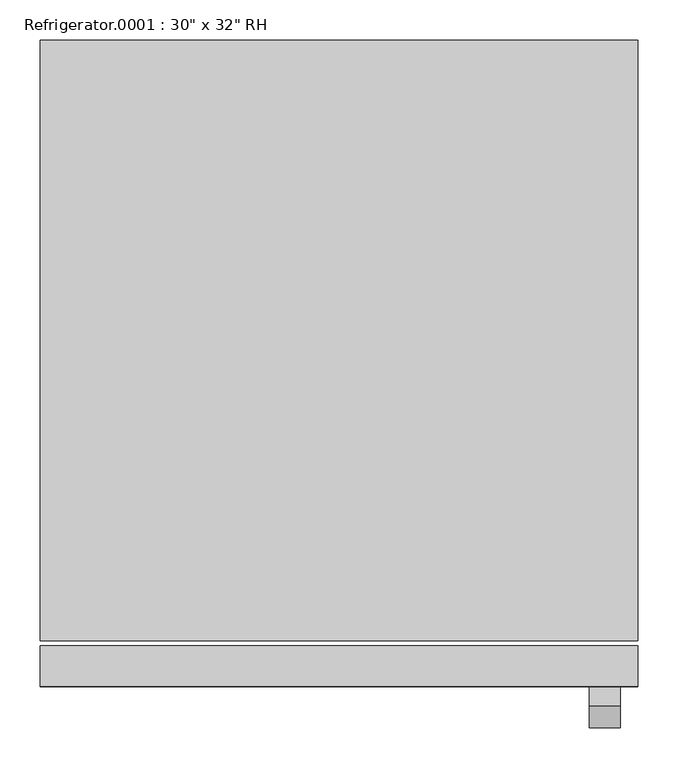
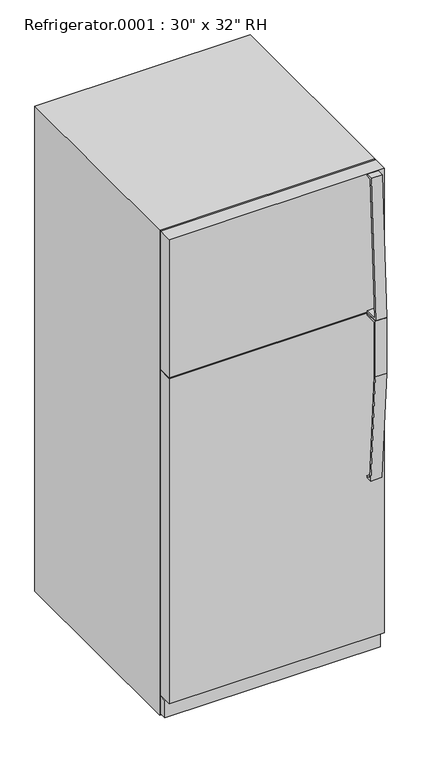
"""IFC4 building model written with IfcOpenShell, lengths in millimetres: proxy geometry."""

from ifc_helpers import new_model, si_unit, frame, origin, origin_with_axes, place, context, project, spatial, polyline, outline, extrude, source, transform, mapped, element, save


def proxy_a13a33b2(model_context):
    return source(origin(), model_context, "Body", "SweptSolid", [
        extrude(outline(polyline([(-417.9010285, 1262.0625), (-462.3510285, 1262.0625), (-462.3510285, 1065.4342469), (-434.8723987, 672.4715334), (-417.9010285, 672.4715334), (-417.9010285, 666.1370017), (-440.7949512, 666.1370017), (-468.7010285, 1065.2125), (-468.7010285, 1268.4125), (-417.9010285, 1268.4125), (-417.9010285, 1262.0625)])), frame((312.7375, 0.0, 0.0), z_axis=(1.0, 0.0, 0.0), x_axis=(0.0, 1.0, 0.0)), (0.0, 0.0, 1.0), 38.4332978),
        extrude(outline(polyline([(-442.739413, 1778.0), (-418.6780855, 1778.0), (-418.6780855, 1771.65), (-437.5263449, 1771.65), (-463.4007207, 1277.9375), (-418.6780855, 1277.9375), (-418.6780855, 1271.5875), (-469.2793675, 1271.5875), (-442.739413, 1778.0)])), frame((312.7375, 0.0, 0.0), z_axis=(1.0, 0.0, 0.0), x_axis=(0.0, 1.0, 0.0)), (0.0, 0.0, 1.0), 38.4332978),
        extrude(outline(polyline([(373.0625, -367.1010285), (373.0625, -392.5010285), (-373.0625, -392.5010285), (-373.0625, -367.1010285), (373.0625, -367.1010285)])), frame((0.0, 0.0, 9.3816357), z_axis=(0.0, 0.0, 1.0), x_axis=(1.0, 0.0, 0.0)), (0.0, 0.0, 1.0), 63.5),
        extrude(outline(polyline([(373.0625, -367.1010285), (373.0625, -417.9010285), (-373.0625, -417.9010285), (-373.0625, -367.1010285), (373.0625, -367.1010285)])), frame((0.0, 0.0, 76.2), z_axis=(0.0, 0.0, 1.0), x_axis=(1.0, 0.0, 0.0)), (0.0, 0.0, 1.0), 1192.2125),
        extrude(outline(polyline([(373.0625, -367.1010285), (373.0625, -417.9010285), (-373.0625, -417.9010285), (-373.0625, -367.1010285), (373.0625, -367.1010285)])), frame((0.0, 0.0, 1271.5875), z_axis=(0.0, 0.0, 1.0), x_axis=(1.0, 0.0, 0.0)), (0.0, 0.0, 1.0), 506.4125),
        extrude(outline(polyline([(373.0625, 388.5489715), (373.0625, -360.7510285), (-373.0625, -360.7510285), (-373.0625, 388.5489715), (373.0625, 388.5489715)])), origin_with_axes(), (0.0, 0.0, 1.0), 1778.0),
    ])


if __name__ == "__main__":
    model = new_model("IFC4")
    model_context = context("Model", 3, world=origin())
    ifc_project = project(units=[si_unit("LENGTHUNIT", "METRE", prefix="MILLI")], contexts=[model_context])
    site = spatial("IfcSite", under=ifc_project)
    building = spatial("IfcBuilding", under=site)
    placement = place(None, origin())
    proxy_shape = proxy_a13a33b2(model_context)
    element("IfcBuildingElementProxy", 1, Name="Refrigerator.0001 : 30\" x 32\" RH", ObjectType="Refrigerator.0001 : 30\" x 32\" RH", at=placement, inside=building, context=model_context, shape_type="MappedRepresentation", body=[
        mapped(proxy_shape, transform((0.0, 0.0, 0.0), x_axis=(1.0, 0.0, 0.0), y_axis=(0.0, 1.0, 0.0), z_axis=(0.0, 0.0, 1.0))),
    ])
    save(model, "model.ifc")

# Revit data of these elements
# Type "Refrigerator.0001 : 30\" x 32\" RH"
#   Label = "REF."
#   Assembly Code = "E1090400"
#   Depth = 2' - 7 3/4"
#   Handle = 2' - 3"
#   Height = 5' - 10"
#   Rear Clearance = 0' - 2"
#   Top Door Height = 1' - 8"
#   Width = 2' - 5 3/8"
#   Material = Steel, Paint Finish, Ivory, Glossy
#   Default Elevation = 0
# Element 1 (IfcBuildingElementProxy, "Refrigerator.0001 : 30\" x 32\" RH")
#   Materials on its faces: "Steel, Paint Finish, Ivory, Glossy", "Steel, Chrome Plated"
# Materials
#   "Steel, Paint Finish, Ivory, Glossy": class "Metal", colour RGB 247 247 239, transparency 0, Description = "Steel, paint finish, ivory, glossy", Cost = 0
#   "Steel, Chrome Plated": class "Metal", colour RGB 17 17 17, transparency 0, Description = "Chromiuim plated steel", Cost = 0
